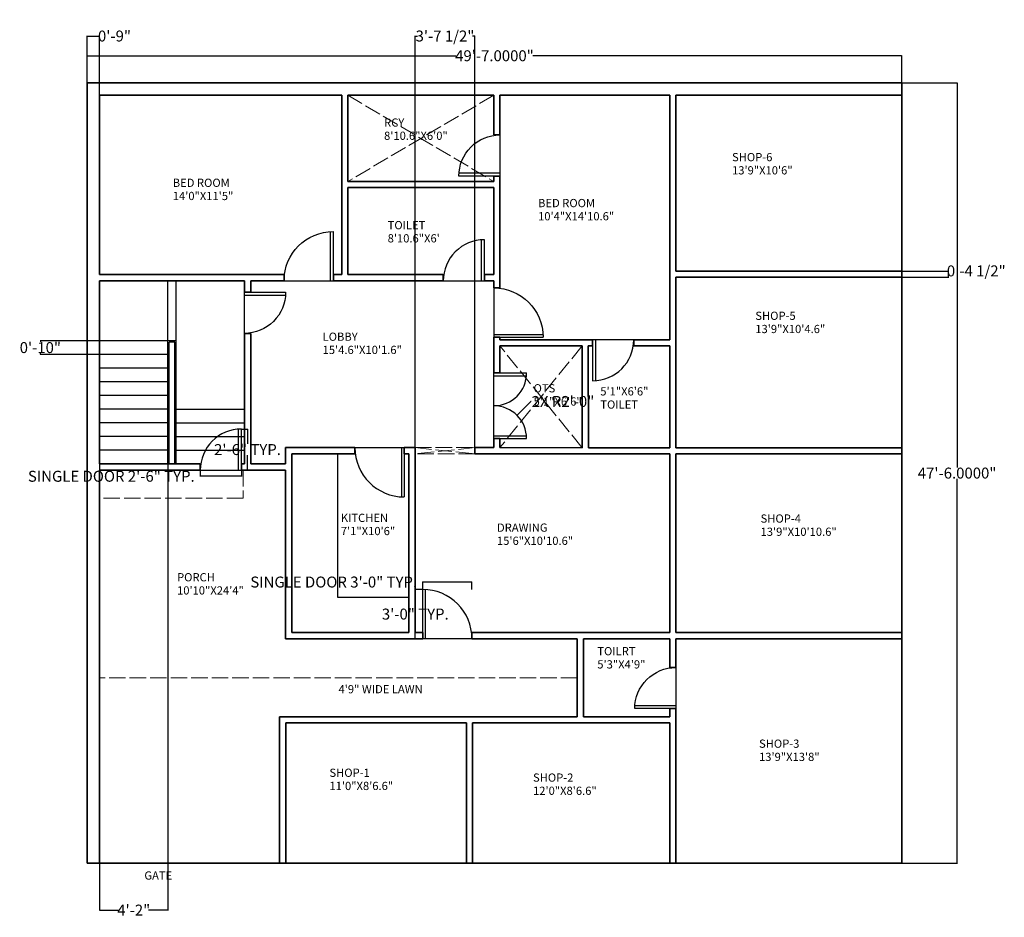
# Model space of a CAD drawing. Units: inches. Extents: x -30 to 689, y 7 to 663.
import ezdxf

# ---------------------------------------------------------------- set-up
doc = ezdxf.new("R2010")
doc.units = ezdxf.units.IN
doc.header["$MEASUREMENT"] = 0
doc.linetypes.add('ACAD_ISO02W100', pattern=[15, 12, -3])
for name, color, linetype, lineweight in [('A-ANNO-DIMS', 2, 'Continuous', 18), ('A-ANNO-TEXT', 7, 'Continuous', 18), ('A-AREA-IDEN', 7, 'Continuous', 18), ('A-DOOR', 4, 'Continuous', 25), ('A-FLOR-FIXT', 8, 'Continuous', 25), ('A-FLOR-OPEN', 8, 'ACAD_ISO02W100', 18), ('A-FLOR-PROJ', 8, 'ACAD_ISO02W100', 18), ('A-FLOR-STRS', 7, 'Continuous', 25), ('A-WALL', 7, 'Continuous', 35), ('A-WALL-OVHD', 7, 'ACAD_ISO02W100', 18), ('C-PROP', 7, 'Continuous', 35), ('L-PLNT', 3, 'ACAD_ISO02W100', 18)]:
    doc.layers.add(name, color=color, linetype=linetype, lineweight=lineweight)
doc.styles.get("Standard").update_dxf_attribs({"font": 'arial.ttf'})
doc.dimstyles.get("Standard").update_dxf_attribs({"dimtxt": 8, "dimasz": 0.18, "dimexe": 0.18, "dimexo": 0.0625, "dimgap": 0.09, "dimtad": 0, "dimtih": 1, "dimtoh": 1, "dimdec": 4, "dimzin": 0, "dimdsep": 46, "dimlunit": 3, "dimtxsty": 'Standard', "dimcen": 0.09, "dimadec": 0, "dimazin": 0, "dimtfac": 1, "dimtdec": 4, "dimtofl": 0, "dimtmove": 0, "dimatfit": 3, "dimfxl": 1, "dimtolj": 1, "dimtzin": 0, "dimarcsym": 0})

# ---------------------------------------------------------------- blocks, each defined once
blk = doc.blocks.new('*D1')
at = {"layer": 'A-ANNO-DIMS', "color": 0, "lineweight": -2, "transparency": 16777216}
for p, q in [((18.9, 616.67), (18.9, 636.63)), ((19.08, 636.45), (288.43, 636.45)), ((613.72, 636.45), (344.38, 636.45)), ((613.9, 616.67), (613.9, 636.63))]:
    blk.add_line(p, q, dxfattribs=at)
at = {"layer": 'A-ANNO-DIMS', "color": 0, "transparency": 16777216}
for points in [[(19.08, 636.48), (19.08, 636.42), (18.9, 636.45)], [(613.72, 636.48), (613.72, 636.42), (613.9, 636.45)]]:
    blk.add_solid(points, dxfattribs=at)
at = {"layer": 'Defpoints', "color": 0, "transparency": 16777216}
for p in [(613.9, 636.45), (18.9, 616.61), (613.9, 616.61)]:
    blk.add_point(p, dxfattribs=at)
at = {"layer": 'A-ANNO-DIMS', "color": 0, "transparency": 16777216, "insert": (316.4, 636.45), "char_height": 8, "attachment_point": 5}
blk.add_mtext('\\A1;49\'-7.0000"', dxfattribs=at)
blk = doc.blocks.new('*D2')
at = {"layer": 'A-ANNO-DIMS', "color": 0, "lineweight": -2, "transparency": 16777216}
for p, q in [((613.96, 616.61), (654.55, 616.61)), ((654.37, 616.43), (654.37, 335.78)), ((654.37, 46.79), (654.37, 327.44)), ((613.96, 46.61), (654.55, 46.61))]:
    blk.add_line(p, q, dxfattribs=at)
at = {"layer": 'A-ANNO-DIMS', "color": 0, "transparency": 16777216}
for points in [[(654.34, 616.43), (654.4, 616.43), (654.37, 616.61)], [(654.34, 46.79), (654.4, 46.79), (654.37, 46.61)]]:
    blk.add_solid(points, dxfattribs=at)
at = {"layer": 'Defpoints', "color": 0, "transparency": 16777216}
for p in [(613.9, 616.61), (613.9, 46.61), (654.37, 46.61)]:
    blk.add_point(p, dxfattribs=at)
at = {"layer": 'A-ANNO-DIMS', "color": 0, "transparency": 16777216, "insert": (654.37, 331.61), "char_height": 8, "attachment_point": 5}
blk.add_mtext('\\A1;47\'-6.0000"', dxfattribs=at)
blk = doc.blocks.new('DOOR-SINGLE-30IN')
for p, q in [((30, 0), (0, 0)), ((0, 0), (0, -30)), ((2, 0), (2, -30))]:
    blk.add_line(p, q)
blk.add_arc((0, 0), 30, 270, 0)
blk = doc.blocks.new('DOOR-SINGLE-36IN')
for p, q in [((-36, 0), (0, 0)), ((-2, 0), (-2, -36)), ((0, 0), (0, -36))]:
    blk.add_line(p, q)
blk.add_arc((0, 0), 36, 180, 270)
blk = doc.blocks.new('*D5')
at = {"layer": 'A-ANNO-DIMS', "color": 0, "lineweight": -2, "transparency": 16777216}
for p, q in [((101.49, 333.72), (101.49, 329.1)), ((131.49, 333.72), (131.49, 329.1)), ((101.49, 329.28), (101.31, 329.28)), ((131.31, 329.28), (101.67, 329.28))]:
    blk.add_line(p, q, dxfattribs=at)
at = {"layer": 'A-ANNO-DIMS', "color": 0, "transparency": 16777216}
for points in [[(101.67, 329.31), (101.67, 329.25), (101.49, 329.28)], [(131.31, 329.31), (131.31, 329.25), (131.49, 329.28)]]:
    blk.add_solid(points, dxfattribs=at)
at = {"layer": 'Defpoints', "color": 0, "transparency": 16777216}
for p in [(101.49, 333.78), (131.49, 333.78), (101.49, 329.28)]:
    blk.add_point(p, dxfattribs=at)
at = {"layer": 'A-ANNO-DIMS', "color": 0, "transparency": 16777216, "insert": (36.49, 329.28), "char_height": 8, "attachment_point": 5}
blk.add_mtext('\\A1;SINGLE DOOR 2\'-6" TYP.', dxfattribs=at)
blk = doc.blocks.new('*D6')
at = {"layer": 'A-ANNO-DIMS', "color": 0, "lineweight": -2, "transparency": 16777216}
for p, q in [((131.55, 363.78), (136.17, 363.78)), ((135.99, 363.6), (135.99, 352.95)), ((135.99, 333.96), (135.99, 344.6)), ((131.55, 333.78), (136.17, 333.78))]:
    blk.add_line(p, q, dxfattribs=at)
at = {"layer": 'A-ANNO-DIMS', "color": 0, "transparency": 16777216}
for points in [[(135.96, 363.6), (136.02, 363.6), (135.99, 363.78)], [(135.96, 333.96), (136.02, 333.96), (135.99, 333.78)]]:
    blk.add_solid(points, dxfattribs=at)
at = {"layer": 'Defpoints', "color": 0, "transparency": 16777216}
for p in [(131.49, 363.78), (131.49, 333.78), (135.99, 333.78)]:
    blk.add_point(p, dxfattribs=at)
at = {"layer": 'A-ANNO-DIMS', "color": 0, "transparency": 16777216, "insert": (135.99, 348.78), "char_height": 8, "attachment_point": 5}
blk.add_mtext('\\A1;2\'-6" TYP.', dxfattribs=at)
blk = doc.blocks.new('*D7')
at = {"layer": 'A-ANNO-DIMS', "color": 0, "lineweight": -2, "transparency": 16777216}
for p, q in [((263.96, 252.01), (263.78, 252.01)), ((263.96, 246.67), (263.96, 252.19)), ((299.78, 252.01), (264.14, 252.01)), ((299.96, 246.67), (299.96, 252.19))]:
    blk.add_line(p, q, dxfattribs=at)
at = {"layer": 'A-ANNO-DIMS', "color": 0, "transparency": 16777216}
for points in [[(264.14, 252.04), (264.14, 251.98), (263.96, 252.01)], [(299.78, 252.04), (299.78, 251.98), (299.96, 252.01)]]:
    blk.add_solid(points, dxfattribs=at)
at = {"layer": 'Defpoints', "color": 0, "transparency": 16777216}
for p in [(263.96, 252.01), (263.96, 246.61), (299.96, 246.61)]:
    blk.add_point(p, dxfattribs=at)
at = {"layer": 'A-ANNO-DIMS', "color": 0, "transparency": 16777216, "insert": (198.96, 252.01), "char_height": 8, "attachment_point": 5}
blk.add_mtext('\\A1;SINGLE DOOR 3\'-0" TYP.', dxfattribs=at)
blk = doc.blocks.new('*D8')
at = {"layer": 'A-ANNO-DIMS', "color": 0, "lineweight": -2, "transparency": 16777216}
for p, q in [((263.9, 246.61), (258.38, 246.61)), ((258.56, 246.43), (258.56, 232.79)), ((258.56, 210.79), (258.56, 224.43)), ((263.9, 210.61), (258.38, 210.61))]:
    blk.add_line(p, q, dxfattribs=at)
at = {"layer": 'A-ANNO-DIMS', "color": 0, "transparency": 16777216}
for points in [[(258.53, 246.43), (258.59, 246.43), (258.56, 246.61)], [(258.53, 210.79), (258.59, 210.79), (258.56, 210.61)]]:
    blk.add_solid(points, dxfattribs=at)
at = {"layer": 'Defpoints', "color": 0, "transparency": 16777216}
for p in [(263.96, 246.61), (258.56, 210.61), (263.96, 210.61)]:
    blk.add_point(p, dxfattribs=at)
at = {"layer": 'A-ANNO-DIMS', "color": 0, "transparency": 16777216, "insert": (258.56, 228.61), "char_height": 8, "attachment_point": 5}
blk.add_mtext('\\A1;3\'-0" TYP.', dxfattribs=at)
blk = doc.blocks.new('*D9')
at = {"layer": 'A-ANNO-DIMS', "color": 0, "lineweight": -2, "transparency": 16777216}
for p, q in [((27.9, 338.22), (27.9, 12.18)), ((77.86, 338.22), (77.86, 12.18)), ((28.08, 12.36), (42, 12.36)), ((77.68, 12.36), (63.76, 12.36))]:
    blk.add_line(p, q, dxfattribs=at)
at = {"layer": 'A-ANNO-DIMS', "color": 0, "transparency": 16777216}
for points in [[(28.08, 12.39), (28.08, 12.33), (27.9, 12.36)], [(77.68, 12.39), (77.68, 12.33), (77.86, 12.36)]]:
    blk.add_solid(points, dxfattribs=at)
at = {"layer": 'Defpoints', "color": 0, "transparency": 16777216}
for p in [(27.9, 338.28), (77.86, 338.28), (77.86, 12.36)]:
    blk.add_point(p, dxfattribs=at)
at = {"layer": 'A-ANNO-DIMS', "color": 0, "transparency": 16777216, "insert": (52.88, 12.36), "char_height": 8, "attachment_point": 5}
blk.add_mtext('\\A1;4\'-2"', dxfattribs=at)
blk = doc.blocks.new('*D10')
at = {"layer": 'A-ANNO-DIMS', "color": 0, "lineweight": -2, "transparency": 16777216}
for p, q in [((27.84, 428.28), (-15.53, 428.28)), ((-15.35, 428.1), (-15.35, 427.45)), ((27.84, 418.28), (-15.53, 418.28)), ((-15.35, 418.46), (-15.35, 419.1))]:
    blk.add_line(p, q, dxfattribs=at)
at = {"layer": 'A-ANNO-DIMS', "color": 0, "transparency": 16777216}
for points in [[(-15.38, 428.1), (-15.32, 428.1), (-15.35, 428.28)], [(-15.38, 418.46), (-15.32, 418.46), (-15.35, 418.28)]]:
    blk.add_solid(points, dxfattribs=at)
at = {"layer": 'Defpoints', "color": 0, "transparency": 16777216}
for p in [(27.9, 428.28), (-15.35, 418.28), (27.9, 418.28)]:
    blk.add_point(p, dxfattribs=at)
at = {"layer": 'A-ANNO-DIMS', "color": 0, "transparency": 16777216, "insert": (-15.35, 423.28), "char_height": 8, "attachment_point": 5}
blk.add_mtext('\\A1;0\'-10"', dxfattribs=at)
blk = doc.blocks.new('*D11')
at = {"layer": 'A-ANNO-DIMS', "color": 0, "lineweight": -2, "transparency": 16777216}
for p, q in [((258.4, 350.24), (258.4, 651.04)), ((258.58, 650.86), (260.22, 650.86)), ((301.94, 650.86), (300.3, 650.86)), ((302.12, 350.24), (302.12, 651.04))]:
    blk.add_line(p, q, dxfattribs=at)
at = {"layer": 'A-ANNO-DIMS', "color": 0, "transparency": 16777216}
for points in [[(258.58, 650.89), (258.58, 650.83), (258.4, 650.86)], [(301.94, 650.89), (301.94, 650.83), (302.12, 650.86)]]:
    blk.add_solid(points, dxfattribs=at)
at = {"layer": 'Defpoints', "color": 0, "transparency": 16777216}
for p in [(302.12, 650.86), (258.4, 350.18), (302.12, 350.18)]:
    blk.add_point(p, dxfattribs=at)
at = {"layer": 'A-ANNO-DIMS', "color": 0, "transparency": 16777216, "insert": (280.26, 650.86), "char_height": 8, "attachment_point": 5}
blk.add_mtext('\\A1;3\'-7 1/2"', dxfattribs=at)
blk = doc.blocks.new('*D12')
at = {"layer": 'A-ANNO-DIMS', "color": 0, "lineweight": -2, "transparency": 16777216}
for p, q in [((613.96, 479.11), (648.33, 479.11)), ((648.15, 479.11), (648.15, 479.29)), ((648.15, 479.29), (648.33, 479.29)), ((648.15, 474.79), (648.15, 478.93)), ((613.96, 474.61), (648.33, 474.61))]:
    blk.add_line(p, q, dxfattribs=at)
at = {"layer": 'A-ANNO-DIMS', "color": 0, "transparency": 16777216}
for points in [[(648.12, 478.93), (648.18, 478.93), (648.15, 479.11)], [(648.12, 474.79), (648.18, 474.79), (648.15, 474.61)]]:
    blk.add_solid(points, dxfattribs=at)
at = {"layer": 'Defpoints', "color": 0, "transparency": 16777216}
for p in [(613.9, 479.11), (648.15, 479.11), (613.9, 474.61)]:
    blk.add_point(p, dxfattribs=at)
at = {"layer": 'A-ANNO-DIMS', "color": 0, "transparency": 16777216, "insert": (668.38, 479.29), "char_height": 8, "attachment_point": 5}
blk.add_mtext('\\A1;0\'-4 1/2"', dxfattribs=at)
blk = doc.blocks.new('*D13')
at = {"layer": 'A-ANNO-DIMS', "color": 0, "lineweight": -2, "transparency": 16777216}
for p, q in [((18.9, 616.67), (18.9, 651.04)), ((19.08, 650.86), (27.72, 650.86)), ((27.9, 607.67), (27.9, 651.04)), ((27.9, 650.86), (28.08, 650.86))]:
    blk.add_line(p, q, dxfattribs=at)
at = {"layer": 'A-ANNO-DIMS', "color": 0, "transparency": 16777216}
for points in [[(19.08, 650.89), (19.08, 650.83), (18.9, 650.86)], [(27.72, 650.89), (27.72, 650.83), (27.9, 650.86)]]:
    blk.add_solid(points, dxfattribs=at)
at = {"layer": 'Defpoints', "color": 0, "transparency": 16777216}
for p in [(27.9, 650.86), (18.9, 616.61), (27.9, 607.61)]:
    blk.add_point(p, dxfattribs=at)
at = {"layer": 'A-ANNO-DIMS', "color": 0, "transparency": 16777216, "insert": (38.81, 650.86), "char_height": 8, "attachment_point": 5}
blk.add_mtext('\\A1;0\'-9"', dxfattribs=at)
blk = doc.blocks.new('*D14')
at = {"layer": 'A-ANNO-DIMS', "color": 0, "lineweight": -2, "transparency": 16777216}
for p, q in [((343.06, 383.9), (333, 373.85)), ((343.24, 383.9), (343.06, 383.9)), ((315.81, 356.75), (315.99, 356.75)), ((315.9, 356.66), (315.9, 356.84))]:
    blk.add_line(p, q, dxfattribs=at)
at = {"layer": 'A-ANNO-DIMS', "color": 0, "transparency": 16777216}
blk.add_solid([(332.98, 373.87), (333.02, 373.82), (332.87, 373.72)], dxfattribs=at)
at = {"layer": 'Defpoints', "color": 0, "transparency": 16777216}
for p in [(332.87, 373.72), (315.9, 356.75)]:
    blk.add_point(p, dxfattribs=at)
at = {"layer": 'A-ANNO-DIMS', "color": 0, "transparency": 16777216, "insert": (366.45, 383.9), "char_height": 8, "attachment_point": 5}
blk.add_mtext('\\A1;2X R2\'-0"', dxfattribs=at)

msp = doc.modelspace()

# ---------------------------------------------------------------- linework, layer by layer
at = {"layer": 'A-DOOR'}
for p, q in [((315.90223, 356.74714), (315.90223, 404.74714)), ((315.90223, 404.74714), (339.90223, 404.74714)), ((315.90223, 402.74714), (339.90223, 402.74714)), ((315.90223, 358.74714), (339.90223, 358.74714)), ((315.90223, 356.74714), (339.90223, 356.74714))]:
    msp.add_line(p, q, dxfattribs=at)
for centre, start, end in [((315.90223, 404.74714), 270, 360), ((315.90223, 356.74714), 0, 90)]:
    msp.add_arc(centre, 24, start, end, dxfattribs=at)
at = {"layer": 'A-FLOR-FIXT'}
for p, q in [((201.74474, 345.61019), (201.74474, 240.96434)), ((201.74474, 240.96434), (253.90223, 240.96434))]:
    msp.add_line(p, q, dxfattribs=at)
at = {"layer": 'A-FLOR-OPEN'}
for p, q in [((209.30223, 607.61019), (315.90223, 544.61019)), ((315.90223, 607.61019), (209.30223, 544.61019)), ((380.40223, 350.14472), (320.40223, 424.51019)), ((380.40223, 424.51019), (320.40223, 350.1771))]:
    msp.add_line(p, q, dxfattribs=at)
at = {"layer": 'A-FLOR-PROJ'}
for p, q in [((132.78951, 333.77956), (132.78951, 313.1646)), ((132.78951, 313.1646), (27.90223, 313.1646))]:
    msp.add_line(p, q, dxfattribs=at)
at = {"layer": 'A-FLOR-STRS'}
for p, q in [((77.85606, 338.27956), (77.85606, 472.07594)), ((83.85606, 338.27956), (83.85606, 472.07594)), ((83.85606, 428.27956), (27.90223, 428.27956)), ((82.85606, 427.27956), (78.85606, 427.27956)), ((78.85606, 338.27956), (78.85606, 427.27956)), ((82.85606, 338.27956), (82.85606, 427.27956)), ((77.85606, 418.27956), (27.90223, 418.27956)), ((77.85606, 408.27956), (27.90223, 408.27956)), ((77.85606, 398.27956), (27.90223, 398.27956)), ((77.85606, 388.27956), (27.90223, 388.27956)), ((77.85606, 378.27956), (27.90223, 378.27956)), ((83.85606, 378.27956), (133.8099, 378.27956)), ((77.85606, 368.27956), (27.90223, 368.27956)), ((83.85606, 368.27956), (133.8099, 368.27956)), ((77.85606, 358.27956), (27.90223, 358.27956)), ((83.85606, 358.27956), (133.8099, 358.27956)), ((77.85606, 348.27956), (27.90223, 348.27956)), ((83.85606, 348.27956), (133.8099, 348.27956)), ((77.85606, 338.27956), (27.90223, 338.27956)), ((83.85606, 338.27956), (101.48637, 338.27956))]:
    msp.add_line(p, q, dxfattribs=at)
at = {"layer": 'A-WALL'}
for p, q in [((27.90223, 607.61019), (27.90223, 476.57594)), ((204.80223, 607.61019), (27.90223, 607.61019)), ((204.80223, 476.57594), (204.80223, 607.61019)), ((315.90223, 607.61019), (209.30223, 607.61019)), ((209.30223, 544.61019), (209.30223, 607.61019)), ((315.90223, 578.5699), (315.90223, 607.61019)), ((444.40223, 607.61019), (320.40223, 607.61019)), ((320.40223, 578.5699), (320.40223, 607.61019)), ((444.40223, 429.01019), (444.40223, 607.61019)), ((613.90223, 607.61019), (448.90223, 607.61019)), ((448.90223, 479.11019), (448.90223, 607.61019)), ((320.40223, 578.5699), (315.90223, 578.5699)), ((315.90223, 544.61019), (315.90223, 548.5699)), ((320.40223, 548.5699), (315.90223, 548.5699)), ((320.40223, 466.89639), (320.40223, 548.5699)), ((315.90223, 544.61019), (209.30223, 544.61019)), ((209.30223, 476.57594), (209.30223, 540.11019)), ((315.90223, 540.11019), (209.30223, 540.11019)), ((315.90223, 476.57594), (315.90223, 540.11019)), ((162.70135, 476.57594), (27.90223, 476.57594)), ((162.70135, 476.57594), (162.70135, 472.07594)), ((204.80223, 476.57594), (198.70135, 476.57594)), ((198.70135, 476.57594), (198.70135, 472.07594)), ((279.02295, 476.57594), (209.30223, 476.57594)), ((279.02295, 476.57594), (209.30223, 476.57594)), ((279.02295, 472.07594), (279.02295, 476.57594)), ((315.90223, 476.57594), (309.02295, 476.57594)), ((315.90223, 476.57594), (309.02295, 476.57594)), ((309.02295, 472.07594), (309.02295, 476.57594)), ((448.90223, 479.11019), (613.90223, 479.11019)), ((133.8099, 472.07594), (27.90223, 472.07594)), ((27.90223, 472.07594), (27.90223, 338.27956)), ((133.8099, 463.65939), (133.8099, 472.07594)), ((162.70135, 472.07594), (138.3099, 472.07594)), ((138.3099, 463.65939), (138.3099, 472.07594)), ((279.02295, 472.07594), (198.70135, 472.07594)), ((315.90223, 472.07594), (309.02295, 472.07594)), ((315.90223, 466.89639), (315.90223, 472.07594)), ((448.90223, 474.61019), (613.90223, 474.61019)), ((448.90223, 350.11019), (448.90223, 474.61019)), ((138.3099, 463.65939), (133.8099, 463.65939)), ((315.90223, 466.89639), (320.40223, 466.89639)), ((133.8099, 338.27956), (133.8099, 433.65939)), ((138.3099, 433.65939), (133.8099, 433.65939)), ((138.3099, 338.27956), (138.3099, 433.65939)), ((315.90223, 430.89639), (320.40223, 430.89639)), ((315.90223, 404.74714), (315.90223, 430.89639)), ((320.40223, 429.01019), (320.40223, 430.89639)), ((388.12538, 429.01019), (320.40223, 429.01019)), ((380.40223, 424.51019), (320.40223, 424.51019)), ((320.40223, 404.74714), (320.40223, 424.51019)), ((380.40223, 350.14472), (380.40223, 424.51019)), ((385.17652, 350.14215), (384.90223, 424.51019)), ((388.12538, 424.51019), (384.90223, 424.51019)), ((388.12538, 424.51019), (388.12538, 429.01019)), ((444.40223, 429.01019), (418.12538, 429.01019)), ((418.12538, 424.51019), (418.12538, 429.01019)), ((444.40223, 424.51019), (418.12538, 424.51019)), ((444.40223, 350.11019), (444.40223, 424.51019)), ((315.90223, 404.74714), (320.40223, 404.74714)), ((315.90223, 350.17953), (315.90223, 356.74714)), ((315.90223, 356.74714), (320.40223, 356.74714)), ((320.40223, 350.1771), (320.40223, 356.74714)), ((163.80223, 338.27956), (163.80223, 350.21298)), ((163.80223, 350.17953), (209.30223, 350.17953)), ((168.30223, 350.17953), (168.30223, 350.21298)), ((168.30223, 345.61019), (214.45247, 345.61019)), ((168.30223, 215.11019), (168.30223, 345.61019)), ((209.30223, 350.17953), (214.45247, 350.17953)), ((214.45247, 350.17953), (214.45247, 345.61019)), ((250.45247, 350.17953), (250.45247, 345.61019)), ((250.45247, 350.17953), (258.40223, 350.17953)), ((250.45247, 345.61019), (253.90223, 345.61019)), ((253.90223, 350.17953), (253.90223, 350.21298)), ((253.90223, 215.11019), (253.90223, 345.61019)), ((258.40223, 215.11019), (258.40223, 350.17953)), ((302.12409, 345.61019), (302.12409, 350.17953)), ((302.12409, 350.17953), (315.90223, 350.17953)), ((302.12409, 345.61019), (444.40223, 345.61019)), ((320.40223, 350.1771), (380.40223, 350.14472)), ((385.17652, 350.14215), (444.40223, 350.11019)), ((444.40223, 215.11019), (444.40223, 345.61019)), ((448.90223, 350.11019), (613.90223, 350.11019)), ((448.90223, 345.61019), (613.90223, 345.61019)), ((448.90223, 215.11019), (448.90223, 345.61019)), ((101.48637, 338.27956), (27.90223, 338.27956)), ((101.48637, 333.77956), (101.48637, 338.27956)), ((133.8099, 338.27956), (131.48637, 338.27956)), ((131.48637, 333.77956), (131.48637, 338.27956)), ((131.48637, 338.27956), (133.8099, 338.27956)), ((163.80223, 338.27956), (138.3099, 338.27956)), ((27.90223, 333.77956), (27.90223, 46.61019)), ((101.48637, 333.77956), (27.90223, 333.77956)), ((163.80223, 333.77956), (131.48637, 333.77956)), ((163.80223, 210.61019), (163.80223, 333.77956)), ((163.80223, 210.61019), (263.95892, 210.61019)), ((168.30223, 215.11019), (253.90223, 215.11019)), ((258.40223, 215.11019), (263.95892, 215.11019)), ((263.95892, 210.61019), (263.95892, 215.11019)), ((299.95892, 210.61019), (299.95892, 215.11019)), ((299.95892, 215.11019), (444.40223, 215.11019)), ((299.95892, 210.61019), (376.90223, 210.61019)), ((376.90223, 153.61019), (376.90223, 210.61019)), ((381.40223, 153.61019), (381.40223, 210.61019)), ((381.40223, 210.61019), (444.40223, 210.61019)), ((444.40223, 189.59001), (444.40223, 210.61019)), ((448.90223, 215.11019), (613.90223, 215.11019)), ((448.90223, 215.11019), (613.90223, 215.11019)), ((448.90223, 210.61019), (613.90223, 210.61019)), ((448.90223, 189.59001), (448.90223, 210.61019)), ((448.90223, 189.59001), (444.40223, 189.59001)), ((444.40223, 153.61019), (444.40223, 159.59001)), ((448.90223, 159.59001), (444.40223, 159.59001)), ((448.90223, 149.11019), (448.90223, 159.59001)), ((159.40223, 153.61019), (376.90223, 153.61019)), ((159.40223, 46.61019), (159.40223, 153.61019)), ((381.40223, 153.61019), (444.40223, 153.61019)), ((163.90223, 149.11019), (295.90223, 149.11019)), ((163.90223, 46.61019), (163.90223, 149.11019)), ((295.90223, 46.61019), (295.90223, 149.11019)), ((300.40223, 46.61019), (300.40223, 149.11019)), ((300.40223, 149.11019), (444.40223, 149.11019)), ((444.40223, 46.61019), (444.40223, 149.11019)), ((448.90223, 46.61019), (448.90223, 149.11019))]:
    msp.add_line(p, q, dxfattribs=at)
at = {"layer": 'A-WALL-OVHD'}
for p, q in [((258.40223, 345.61019), (258.40223, 350.17953)), ((258.40223, 350.17953), (302.12409, 350.17953)), ((302.12409, 350.17953), (258.40223, 345.61019)), ((258.40223, 345.61019), (258.40223, 350.17953)), ((258.40223, 350.17953), (302.12409, 345.61019)), ((302.12409, 345.61019), (258.40223, 345.61019))]:
    msp.add_line(p, q, dxfattribs=at)
at = {"layer": 'C-PROP'}
for p, q in [((613.90223, 616.61019), (18.90223, 616.61019)), ((18.90223, 616.61019), (18.90223, 46.61019)), ((613.90223, 46.61019), (613.90223, 616.61019)), ((18.90223, 46.61019), (613.90223, 46.61019))]:
    msp.add_line(p, q, dxfattribs=at)
at = {"layer": 'L-PLNT'}
msp.add_line((376.90223, 182.11019), (27.90223, 182.11019), dxfattribs=at)

# ---------------------------------------------------------------- block references
at = {"layer": 'A-DOOR', "extrusion": (0, 0, -1), "zscale": -1}
for name, p, rotation in [('DOOR-SINGLE-30IN', (-320.40223, 548.5699), 90.00000000000024), ('DOOR-SINGLE-36IN', (-198.70135, 472.07594), 180), ('DOOR-SINGLE-30IN', (-133.8099, 463.65939), 270.0000000000002), ('DOOR-SINGLE-36IN', (-315.90223, 430.89639), 270.0000000000067), ('DOOR-SINGLE-30IN', (-448.90223, 159.59001), 90.00000000000006)]:
    msp.add_blockref(name, p, dxfattribs=dict(at, rotation=rotation))
at = {"layer": 'A-DOOR', "rotation": 180}
for name, p in [('DOOR-SINGLE-30IN', (309.02295, 472.07594)), ('DOOR-SINGLE-30IN', (131.48637, 333.77956)), ('DOOR-SINGLE-36IN', (263.95892, 210.61019))]:
    msp.add_blockref(name, p, dxfattribs=at)
at = {"layer": 'A-DOOR'}
for name, p in [('DOOR-SINGLE-30IN', (388.12538, 429.01019)), ('DOOR-SINGLE-36IN', (250.45247, 350.17953))]:
    msp.add_blockref(name, p, dxfattribs=at)

# ---------------------------------------------------------------- texts
at = {"layer": 'A-ANNO-TEXT'}
msp.add_text('GATE', height=6, dxfattribs=at).set_placement((60.64422, 34.65333))
at = {"layer": 'A-AREA-IDEN'}
for s, p in [('RCY', (235.75011, 584.66368)), ('8\'10.6"X6\'0"', (235.75011, 575.0252)), ('SHOP-6', (489.96439, 559.39353)), ('13\'9"X10\'6"', (489.96439, 549.75506)), ('BED ROOM', (81.39016, 540.65877)), ('14\'0"X11\'5"', (81.39016, 531.0203)), ('BED ROOM', (348.24975, 525.84523)), ('10\'4"X14\'10.6"', (348.24975, 516.20676)), ('TOILET', (238.36639, 509.72462)), ('8\'10.6"X6\'', (238.36639, 500.08615)), ('SHOP-5', (506.97015, 443.49942)), ('13\'9"X10\'4.6"', (506.97015, 433.86095)), ('LOBBY', (190.8683, 428.22282)), ('15\'4.6"X10\'1.6"', (190.8683, 418.58435)), ('OTS', (344.9724, 390.53785)), ('5\'1"X6\'6"', (393.71231, 388.29875)), ('5\'1"X6\'6"', (344.9724, 380.89938)), ('TOILET', (393.71231, 378.66028)), ('KITCHEN', (204.17752, 295.9068)), ('SHOP-4', (510.8084, 295.39621)), ('7\'1"X10\'6"', (204.17752, 286.26833)), ('DRAWING', (318.24518, 288.76991)), ('13\'9"X10\'10.6"', (510.8084, 285.75774)), ('15\'6"X10\'10.6"', (318.24518, 279.13144)), ('PORCH', (84.51942, 252.52162)), ('10\'10"X24\'4"', (84.51942, 242.88315)), ('TOILRT', (391.53339, 198.50654)), ('5\'3"X4\'9"', (391.53339, 188.86807)), ('4\'9" WIDE LAWN', (202.49423, 170.74676)), ('SHOP-3', (509.68296, 130.94184)), ('13\'9"X13\'8"', (509.68296, 121.30337)), ('SHOP-1', (195.8547, 109.71256)), ('SHOP-2', (344.58008, 106.17434)), ('11\'0"X8\'6.6"', (195.8547, 100.07408)), ('12\'0"X8\'6.6"', (344.58008, 96.53587))]:
    msp.add_text(s, height=6, dxfattribs=at).set_placement(p)

# ---------------------------------------------------------------- dimensions: what is measured, and where the dimension line sits
at = {"layer": 'A-ANNO-DIMS'}
for base, p1, p2, override, picture, middle in [((302.12409, 650.86019), (258.40223, 350.17953), (302.12409, 350.17953), {"dimdec": 1, "dimlfac": 1, "dimrnd": 0, "dimzin": 1, "dimdsep": 46, "dimlunit": 4, "dimfrac": 2}, '*D11', (280.26316, 650.86019)), ((27.90223, 650.86019), (18.90223, 616.61019), (27.90223, 607.61019), {"dimdec": 1, "dimlfac": 1, "dimrnd": 0, "dimzin": 1, "dimdsep": 46, "dimlunit": 4, "dimfrac": 2}, '*D13', (38.80525, 650.86019)), ((613.90223, 636.44557), (18.90223, 616.61019), (613.90223, 616.61019), {"dimclrd": 0, "dimclre": 0, "dimclrt": 0}, '*D1', (316.40223, 636.44557)), ((77.85606, 12.36019), (27.90223, 338.27956), (77.85606, 338.27956), {"dimdec": 1, "dimlfac": 1, "dimrnd": 0, "dimzin": 1, "dimdsep": 46, "dimlunit": 4, "dimfrac": 2}, '*D9', (52.87915, 12.36019))]:
    dim = msp.add_linear_dim(base=base, p1=p1, p2=p2, dimstyle='Standard', override=override, dxfattribs=at)
    dim.commit()
    dim.dimension.update_dxf_attribs({"geometry": picture, "text_midpoint": middle})
for base, p1, p2, override, picture, middle in [((654.37323, 46.61019), (613.90223, 616.61019), (613.90223, 46.61019), {"dimclrd": 0, "dimclre": 0, "dimclrt": 0}, '*D2', (654.37323, 331.61019)), ((648.15223, 479.11019), (613.90223, 474.61019), (613.90223, 479.11019), {"dimdec": 1, "dimlfac": 1, "dimrnd": 0, "dimzin": 1, "dimdsep": 46, "dimlunit": 4, "dimfrac": 2}, '*D12', (668.37585, 479.29019)), ((-15.34777, 418.27956), (27.90223, 428.27956), (27.90223, 418.27956), {"dimdec": 1, "dimlfac": 1, "dimrnd": 0, "dimzin": 1, "dimdsep": 46, "dimlunit": 4, "dimfrac": 2}, '*D10', (-15.34777, 423.27956))]:
    dim = msp.add_linear_dim(base=base, p1=p1, p2=p2, angle=90, dimstyle='Standard', override=override, dxfattribs=at)
    dim.commit()
    dim.dimension.update_dxf_attribs({"geometry": picture, "text_midpoint": middle})
dim = msp.add_radius_dim(center=(315.90223, 356.74714), mpoint=(332.87275, 373.71775), text='2X <>', dimstyle='Standard', override={"dimdec": 1, "dimlfac": 1, "dimrnd": 0, "dimzin": 1, "dimdsep": 46, "dimlunit": 4, "dimfrac": 2}, dxfattribs=at)
dim.commit()
dim.dimension.update_dxf_attribs({"geometry": '*D14', "text_midpoint": (366.4492, 383.90011), "dimtype": 164})
for base, p1, p2, angle, text, picture, middle in [((135.98637, 333.77956), (131.48637, 363.77956), (131.48637, 333.77956), 270, '<> TYP.', '*D6', (135.98637, 348.77956)), ((101.48637, 329.27956), (131.48637, 333.77956), (101.48637, 333.77956), 180, 'SINGLE DOOR <> TYP.', '*D5', (36.48786, 329.27956)), ((263.95892, 252.01019), (299.95892, 246.61019), (263.95892, 246.61019), 180, 'SINGLE DOOR <> TYP.', '*D7', (198.96041, 252.01019)), ((258.55892, 210.61019), (263.95892, 246.61019), (263.95892, 210.61019), 270, '<> TYP.', '*D8', (258.55892, 228.61019))]:
    dim = msp.add_linear_dim(base=base, p1=p1, p2=p2, angle=angle, text=text, dimstyle='Standard', override={"dimdec": 1, "dimlfac": 1, "dimrnd": 0, "dimzin": 1, "dimdsep": 46, "dimlunit": 4, "dimfrac": 2}, dxfattribs=at)
    dim.commit()
    dim.dimension.update_dxf_attribs({"geometry": picture, "text_midpoint": middle})

doc.saveas('drawing.dxf')
